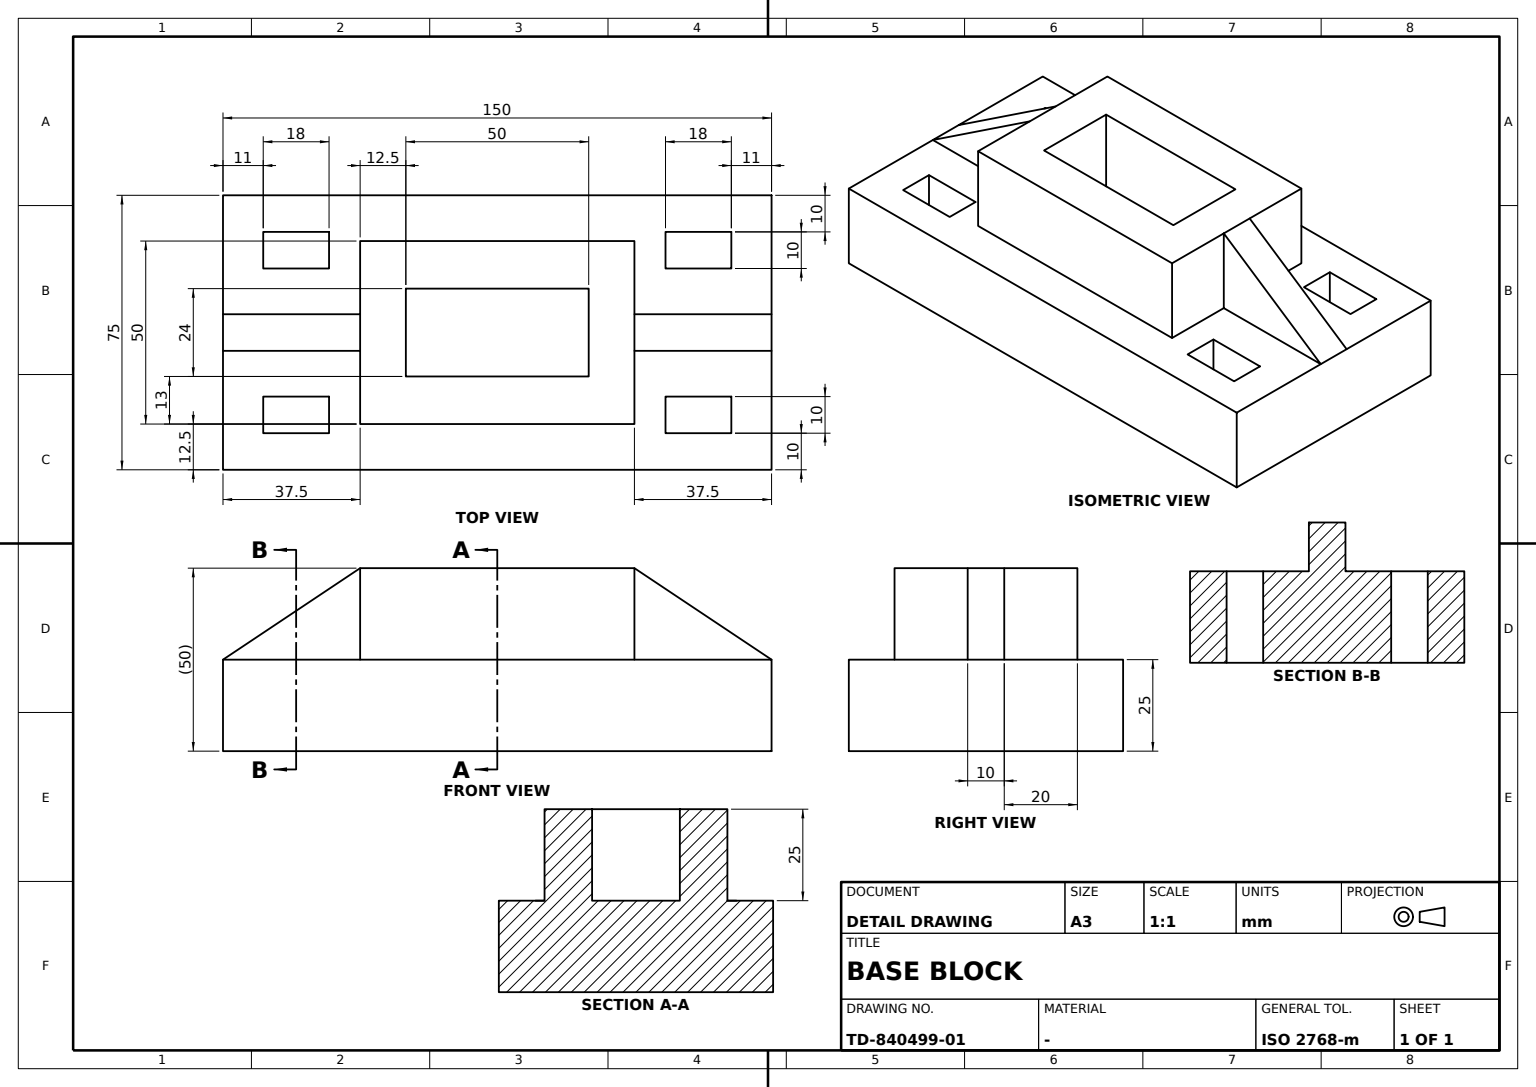
CATIA V5 part; units mm, degrees
sketch "Sketch1" plane through (0, 0, 0) normal (0, 0, 1) x (1, 0, 0)
  line L0 (75, 37.5) -> (75, -37.5)
  line L1 (75, -37.5) -> (-75, -37.5)
  line L2 (-75, -37.5) -> (-75, 37.5)
  line L3 (-75, 37.5) -> (75, 37.5)
  dimension "length L0" = 75
  dimension "length L1" = 150
  constraint vertical L0 y-axis
  constraint vertical L2 y-axis
  constraint horizontal L1 x-axis
  constraint horizontal L3 x-axis
  constraint equidistance L0 L2 origin
  constraint equidistance L1 L3 origin
extrude "Pad1" add sketch "Sketch1" along normal blind 25
sketch "Sketch2" plane through (0, 0, 25) normal (0, 0, 1) x (1, 0, 0)
  point P0 (55, 22.5)
  line L0 (64, 27.5) -> (64, 17.5)
  line L1 (64, 17.5) -> (46, 17.5)
  line L2 (46, 17.5) -> (46, 27.5)
  line L3 (46, 27.5) -> (64, 27.5)
  point P1 (55, -22.5)
  line L4 (64, -17.5) -> (64, -27.5)
  line L5 (64, -27.5) -> (46, -27.5)
  line L6 (46, -27.5) -> (46, -17.5)
  line L7 (46, -17.5) -> (64, -17.5)
  point P2 (64, -27.5)
  line L8 (75, -37.5) -> (75, 37.5) construction
  line L9 (-75, -37.5) -> (75, -37.5) construction
  line L10 (75, 37.5) -> (-75, 37.5) construction
  point P3 (-55, 22.5)
  line L11 (-46, 27.5) -> (-46, 17.5)
  line L12 (-46, 17.5) -> (-64, 17.5)
  line L13 (-64, 17.5) -> (-64, 27.5)
  line L14 (-64, 27.5) -> (-46, 27.5)
  point P4 (-55, -22.5)
  line L15 (-46, -17.5) -> (-46, -27.5)
  line L16 (-46, -27.5) -> (-64, -27.5)
  line L17 (-64, -27.5) -> (-64, -17.5)
  line L18 (-64, -17.5) -> (-46, -17.5)
  point P5 (-46, -27.5)
  line L19 (-75, 37.5) -> (-75, -37.5) construction
  line L20 (75, 37.5) -> (-75, 37.5) construction
  line L21 (-75, -37.5) -> (75, -37.5) construction
  dimension "distance P1 L8" = 20
  dimension "length L7" = 18
  dimension "length L6" = 10
  dimension "distance L9 P1" = 15
  dimension "length L3" = 18
  dimension "length L2" = 10
  dimension "distance L10 P0" = 15
  dimension "length L14" = 18
  dimension "distance P3 L19" = 20
  dimension "distance L20 P3" = 15
  dimension "length L11" = 10
  dimension "length L18" = 18
  dimension "distance P4 L21" = 15
  constraint vertical L0 y-axis
  constraint vertical L2 y-axis
  constraint vertical L4 y-axis
  constraint vertical L6 y-axis
  constraint vertical L11 y-axis
  constraint vertical L13 y-axis
  constraint vertical L15 y-axis
  constraint vertical L17 y-axis
  constraint horizontal L1 x-axis
  constraint horizontal L3 x-axis
  constraint horizontal L5 x-axis
  constraint horizontal L7 x-axis
  constraint horizontal L12 x-axis
  constraint horizontal L14 x-axis
  constraint horizontal L16 x-axis
  constraint horizontal L18 x-axis
  constraint equidistance L0 L2 P0
  constraint equidistance L1 L3 P0
  constraint equidistance L4 L6 P1
  constraint equidistance L5 L7 P1
  constraint equidistance L11 L13 P3
  constraint equidistance L12 L14 P3
  constraint equidistance L15 L17 P4
  constraint equidistance L16 L18 P4
  constraint coincidence P2 L0
  constraint coincidence P5 L11
  constraint coincidence P5 L5
extrude "Pocket1" cut sketch "Sketch2" against normal blind 25
sketch "Sketch3" plane through (0, 0, 25) normal (0, 0, 1) x (1, 0, 0)
  line L0 (25, 12) -> (25, -12)
  line L1 (25, -12) -> (-25, -12)
  line L2 (-25, -12) -> (-25, 12)
  line L3 (-25, 12) -> (25, 12)
  line L4 (37.5, 25) -> (37.5, -25)
  line L5 (37.5, -25) -> (-37.5, -25)
  line L6 (-37.5, -25) -> (-37.5, 25)
  line L7 (-37.5, 25) -> (37.5, 25)
  dimension "length L3" = 50
  dimension "length L5" = 75
  dimension "length L0" = 24
  dimension "length L4" = 50
  constraint vertical L0 y-axis
  constraint vertical L2 y-axis
  constraint vertical L4 y-axis
  constraint vertical L6 y-axis
  constraint horizontal L1 x-axis
  constraint horizontal L3 x-axis
  constraint horizontal L5 x-axis
  constraint horizontal L7 x-axis
  constraint equidistance L0 L2 origin
  constraint equidistance L1 L3 origin
  constraint equidistance L4 L6 origin
  constraint equidistance L5 L7 origin
extrude "Pad2" add sketch "Sketch3" along normal blind 25
sketch "Sketch4" plane through (0, 0, 0) normal (0, 1, 0) x (-1, 0, 0)
  point P0 (37.5, 50)
  line L0 (37.5, 50) -> (37.5, 25)
  line L1 (37.5, 25) -> (75, 25)
  point P1 (75, 25)
  line L2 (75, 25) -> (37.5, 50)
  point P2 (37.5, 50)
  point P3 (75, 25)
  constraint vertical L0 y-axis
  constraint horizontal L1 x-axis
  constraint coincidence P2 P0
  constraint coincidence P1 P3
extrude "Pad3" add sketch "Sketch4" along normal mid plane 10
sketch "Sketch5" plane through (0, 0, 0) normal (0, 1, 0) x (-1, 0, 0)
  point P0 (-75, 25)
  line L0 (-75, 25) -> (-37.5, 25)
  line L1 (-37.5, 25) -> (-37.5, 50)
  point P1 (-37.5, 50)
  line L2 (-37.5, 50) -> (-75, 25)
  point P2 (-37.5, 50)
  point P3 (-75, 25)
  constraint horizontal L0 x-axis
  constraint vertical L1 y-axis
  constraint coincidence P1 P2
  constraint coincidence P0 P3
extrude "Pad4" add sketch "Sketch5" along normal mid plane 10
